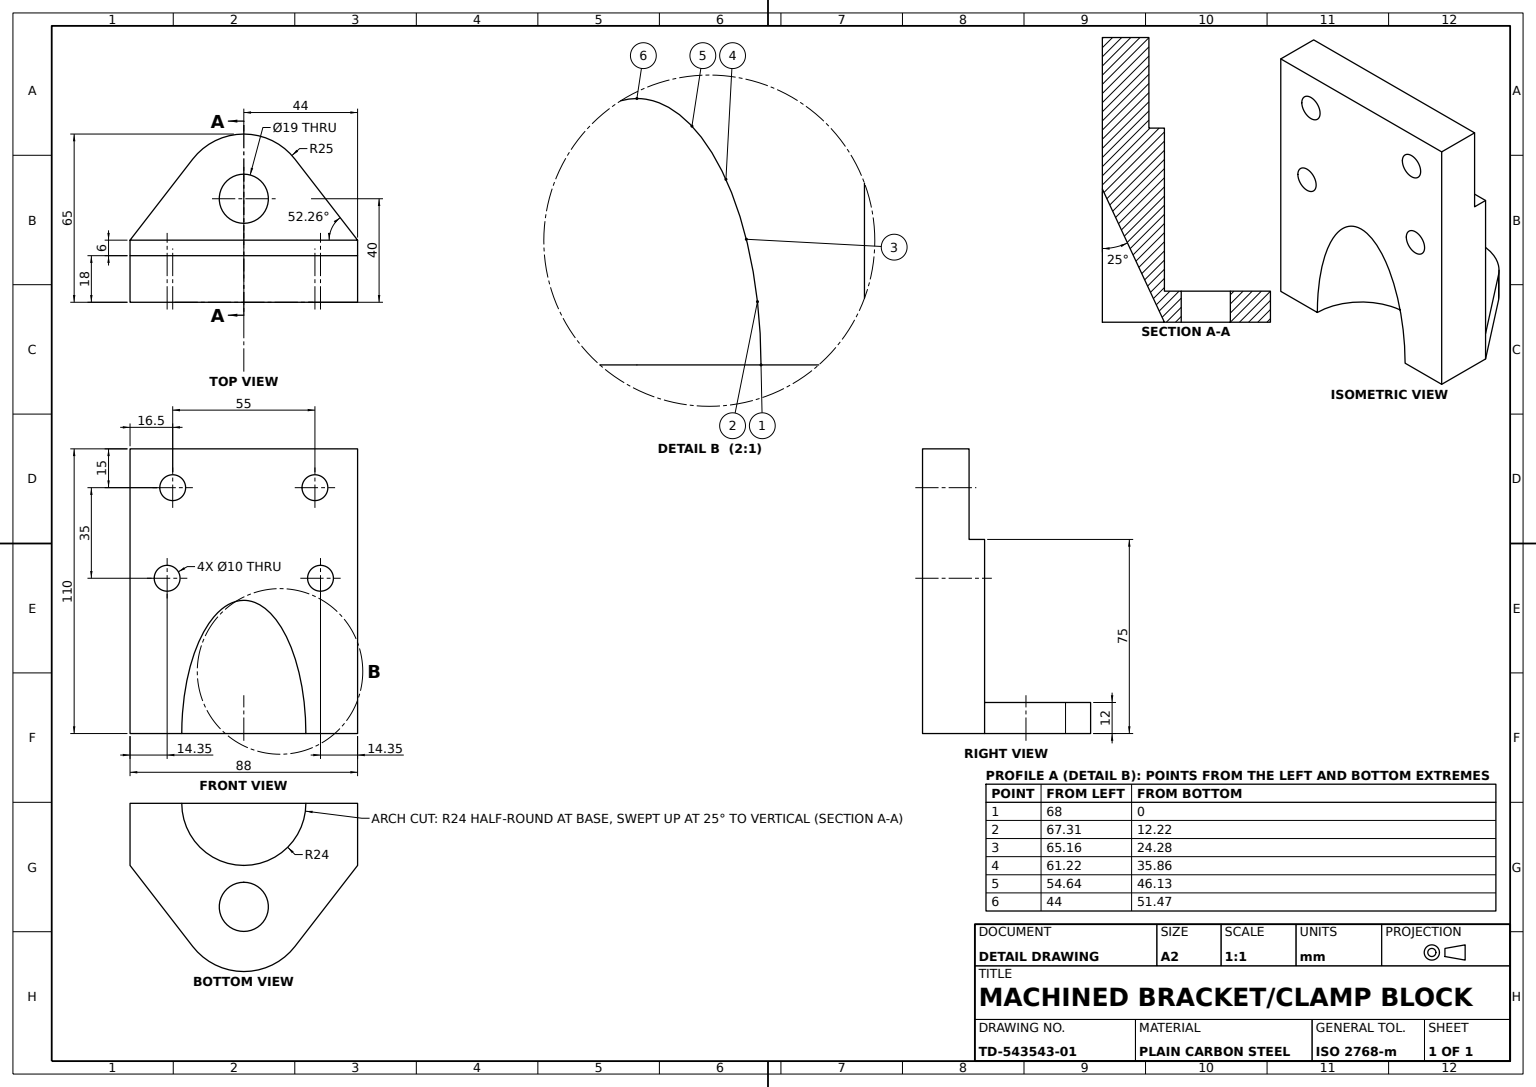
from build123d import *

# Parameters (mm, degrees)
BASE_PLATE_SKETCH_W = 88
BASE_PLATE_SKETCH_H = 110
BASE_PLATE_DEPTH    = 18
SIDE_BOSS_SKETCH_W  = 88
SIDE_BOSS_SKETCH_H  = 6
SIDE_BOSS_DEPTH     = 75
REAR_BOSS_SKETCH_R  = 9.5
REAR_BOSS_DEPTH     = 12
ANGLED_CUT_REACH    = 137.133
ANGLED_CUT_SKETCH_R = 5
ARCH_CUT_SKETCH_R   = 24
ARCH_CUT_DEPTH      = 93.743251702


with BuildPart() as part:
    # Base Plate Sketch → Base Plate (new body)
    with BuildSketch(Plane.XY):
        with Locations((0, 55)):
            Rectangle(BASE_PLATE_SKETCH_W, BASE_PLATE_SKETCH_H)
    extrude(amount=-BASE_PLATE_DEPTH)

    # Side Boss Sketch → Side Boss (add)
    with BuildSketch(Plane(origin=(0, 0, 0), x_dir=(1, 0, 0), z_dir=(0, 1, 0))):
        with Locations((0, 21)):
            Rectangle(SIDE_BOSS_SKETCH_W, SIDE_BOSS_SKETCH_H)
    extrude(amount=SIDE_BOSS_DEPTH)

    # Rear Boss Sketch → Rear Boss (add)
    with BuildSketch(Plane.XZ):
        with BuildLine():
            Line((-44, -24), (-19.769224603, -55.302867659))
            ThreePointArc((-19.769224603, -55.302867659), (0, -65), (19.769224603, -55.302867659))
            Line((19.769224603, -55.302867659), (44, -24))
            Line((44, -24), (-44, -24))
        make_face()
        with Locations(Location((0, -40, 0), (0, 0, 270))):
            Circle(REAR_BOSS_SKETCH_R, mode=Mode.SUBTRACT)
    extrude(amount=-REAR_BOSS_DEPTH)

    # Angled Cut: up to this face of the body (flat: up to its plane)
    angled_cut_end = Plane(part.part.faces().sort_by_distance((0, 43.5, -24))[0])
    # Angled Cut Sketch → Angled Cut (cut, up to the picked face)
    with BuildSketch(Plane.XY, mode=Mode.PRIVATE) as angled_cut_sk1:
        with Locations((-27.5, 95)):
            Circle(ANGLED_CUT_SKETCH_R)
    angled_cut_tool1 = split(extrude(angled_cut_sk1.sketch, amount=-ANGLED_CUT_REACH, mode=Mode.PRIVATE), bisect_by=angled_cut_end, keep=Keep.BOTH, mode=Mode.PRIVATE)
    # Angled Cut Sketch → Angled Cut (cut, up to the picked face)
    with BuildSketch(Plane.XY, mode=Mode.PRIVATE) as angled_cut_sk2:
        with Locations((27.5, 95)):
            Circle(ANGLED_CUT_SKETCH_R)
    angled_cut_tool2 = split(extrude(angled_cut_sk2.sketch, amount=-ANGLED_CUT_REACH, mode=Mode.PRIVATE), bisect_by=angled_cut_end, keep=Keep.BOTH, mode=Mode.PRIVATE)
    # Angled Cut Sketch → Angled Cut (cut, up to the picked face)
    with BuildSketch(Plane.XY, mode=Mode.PRIVATE) as angled_cut_sk3:
        with Locations((29.652920455, 60)):
            Circle(ANGLED_CUT_SKETCH_R)
    angled_cut_tool3 = split(extrude(angled_cut_sk3.sketch, amount=-ANGLED_CUT_REACH, mode=Mode.PRIVATE), bisect_by=angled_cut_end, keep=Keep.BOTH, mode=Mode.PRIVATE)
    # Angled Cut Sketch → Angled Cut (cut, up to the picked face)
    with BuildSketch(Plane.XY, mode=Mode.PRIVATE) as angled_cut_sk4:
        with Locations((-29.652920455, 60)):
            Circle(ANGLED_CUT_SKETCH_R)
    angled_cut_tool4 = split(extrude(angled_cut_sk4.sketch, amount=-ANGLED_CUT_REACH, mode=Mode.PRIVATE), bisect_by=angled_cut_end, keep=Keep.BOTH, mode=Mode.PRIVATE)
    add(angled_cut_tool1.solids().sort_by(Axis((-27.5, 95, 0), (0, 0, -1)))[0], mode=Mode.SUBTRACT)
    add(angled_cut_tool2.solids().sort_by(Axis((27.5, 95, 0), (0, 0, -1)))[0], mode=Mode.SUBTRACT)
    add(angled_cut_tool3.solids().sort_by(Axis((29.65292, 60, 0), (0, 0, -1)))[0], mode=Mode.SUBTRACT)
    add(angled_cut_tool4.solids().sort_by(Axis((-29.65292, 60, 0), (0, 0, -1)))[0], mode=Mode.SUBTRACT)

    # Arch Cut Sketch → Arch Cut (cut, along a direction that is not the sketch's normal)
    with BuildSketch(Plane.XZ):
        Circle(ARCH_CUT_SKETCH_R)
    extrude(amount=-ARCH_CUT_DEPTH, dir=(0, -0.9063077870366493, -0.4226182617407009), mode=Mode.SUBTRACT)


solid = part.part
